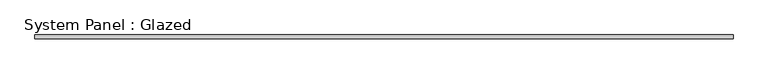
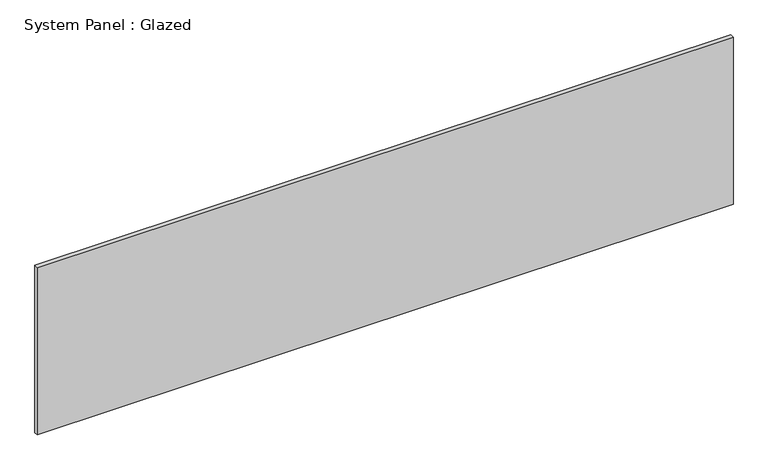
"""IFC4 building model written with IfcOpenShell, lengths in millimetres: plate geometry, System Panel : Glazed."""

from ifc_helpers import new_model, si_unit, origin, origin_with_axes, place, context, project, spatial, polyline, outline, extrude, source, transform, mapped, element, save


def system_panel_glazed_2b5622e6(model_context):
    return source(origin(), model_context, "Body", "SweptSolid", [
        extrude(outline(polyline([(2272.925247, 19.05), (-2272.925247, 19.05), (-2272.925247, 44.45), (2272.925247, 44.45), (2272.925247, 19.05)])), origin_with_axes(), (0.0, 0.0, 1.0), 1155.7),
    ])


if __name__ == "__main__":
    model = new_model("IFC4")
    model_context = context("Model", 3, world=origin())
    ifc_project = project(units=[si_unit("LENGTHUNIT", "METRE", prefix="MILLI")], contexts=[model_context])
    site = spatial("IfcSite", under=ifc_project)
    building = spatial("IfcBuilding", under=site)
    placement = place(None, origin())
    system_panel_glazed_shape = system_panel_glazed_2b5622e6(model_context)
    element("IfcPlate", 1, ObjectType="System Panel : Glazed", at=placement, inside=building, context=model_context, shape_type="MappedRepresentation", body=[
        mapped(system_panel_glazed_shape, transform((0.0, 0.0, 0.0), x_axis=(1.0, 0.0, 0.0), y_axis=(0.0, 1.0, 0.0), z_axis=(0.0, 0.0, 1.0))),
    ])
    save(model, "model.ifc")

# Revit data of these elements
# Type "System Panel : Glazed"
#   Construction Type Id = "GSP4R"
#   Analytic Construction = "1/8 in Pilkington single glazing"
#   Visual Light Transmittance = 0.9
#   Solar Heat Gain Coefficient = 0.86
#   Heat Transfer Coefficient (U) = 1.18115 BTU/(h·ft²·°F)
# Element 1 (IfcPlate, "System Panel : Glazed")
#   Materials on its faces: "Glass"
# Materials
#   "Glass": class "Glass", colour RGB 0 128 192, transparency 0.75, Description = "Soda Lime Glass", Cost = 0
